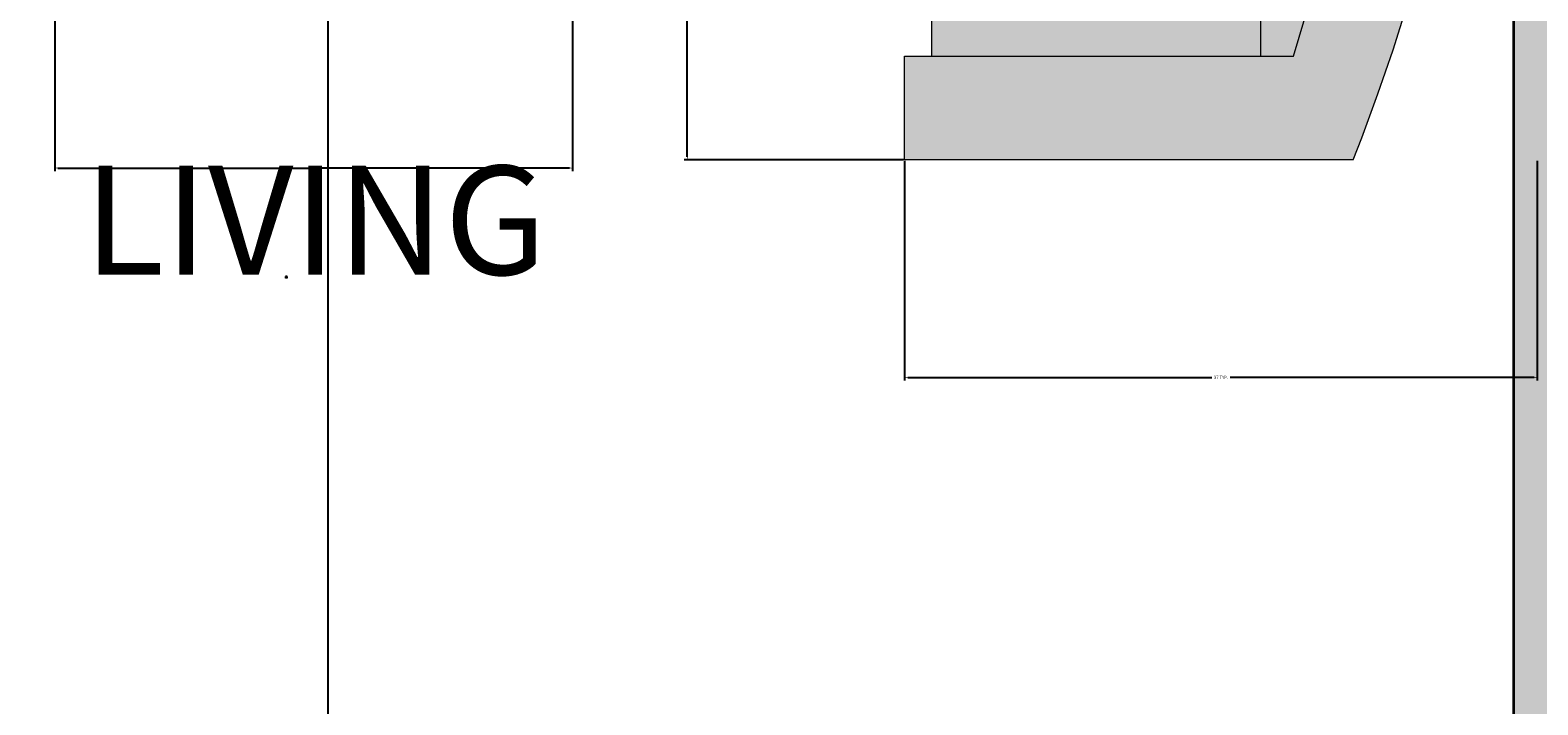
# Model space of a CAD drawing. Units: inches. Extents: x 2549 to 3108, y 1683 to 2362.
# Tile 23 of 30: x 2949 to 3036, y 1979 to 2018. Entities that reach past the tile are written whole.
import ezdxf

# ---------------------------------------------------------------- set-up
doc = ezdxf.new("R2010")
doc.units = ezdxf.units.IN
for name, color, linetype, lineweight in [('A-ANNO-DIMS', 2, 'Continuous', 18), ('A-AREA-IDEN', 7, 'Continuous', 18), ('A-FURN', 8, 'Continuous', 18), ('A-FURN-PATT', 9, 'Continuous', 13), ('A-WALL', 7, 'Continuous', 35), ('A-WALL-PATT', 89, 'Continuous', 13)]:
    doc.layers.add(name, color=color, linetype=linetype, lineweight=lineweight)
doc.layers.add('C-PKNG-VEHI-PATT', color=251, linetype='Continuous', lineweight=13, true_color=0x636466)
doc.layers.add('C-PVMT-PATT', color=9, linetype='Continuous', lineweight=13, true_color=0xc7c8ca)
doc.styles.get("Standard").update_dxf_attribs({"font": 'arial.ttf'})
doc.dimstyles.get("Standard").update_dxf_attribs({"dimtxt": 0.18, "dimasz": 0.18, "dimexe": 0.18, "dimexo": 0.0625, "dimgap": 0.09, "dimtad": 0, "dimtih": 1, "dimtoh": 1, "dimdec": 4, "dimzin": 0, "dimdsep": 46, "dimtxsty": 'Standard', "dimcen": 0.09, "dimadec": 0, "dimazin": 0, "dimtfac": 1, "dimtdec": 4, "dimtofl": 0, "dimtmove": 0, "dimatfit": 3, "dimfxl": 1, "dimtolj": 1, "dimtzin": 0, "dimarcsym": 0})

# ---------------------------------------------------------------- blocks, each defined once
blk = doc.blocks.new('Sofa - Roundback 7 ft.')
for p, q in [((-12.00002, -32.4421), (-12.00003, -6.5971)), ((11.99997, -32.4421), (11.99998, -6.5971)), ((-36.000027, -34), (-36.000027, -11.4696)), ((35.99998, -34), (35.99998, -11.4696)), ((-35.999844, -13.3819), (35.9998, -13.3819)), ((-36.000027, -32.4421), (35.99998, -32.4421))]:
    blk.add_line(p, q)
for points in [[(-36.000027, -34), (-42.000027, -34), (-42.000027, -8)], [(41.99998, -8), (41.99998, -34), (35.99998, -34)]]:
    blk.add_lwpolyline(points)
for centre, radius, start, end in [((0, -114.25), 114.25, 68.43141, 111.5686), ((-0.00001, -127.1968), 121.1968, 72.72033, 107.2797)]:
    blk.add_arc(centre, radius, start, end)
blk = doc.blocks.new('*D16')
at = {"layer": 'A-ANNO-DIMS', "color": 0, "lineweight": -2, "transparency": 16777216}
for p, q in [((2999.284, 2094.091), (2986.567, 2094.091)), ((2986.747, 2093.911), (2986.747, 2052.274)), ((2986.747, 2010.271), (2986.747, 2051.907)), ((2999.284, 2010.091), (2986.567, 2010.091))]:
    blk.add_line(p, q, dxfattribs=at)
at = {"layer": 'A-ANNO-DIMS', "color": 0, "transparency": 16777216}
for points in [[(2986.717, 2093.911), (2986.777, 2093.911), (2986.747, 2094.091)], [(2986.717, 2010.271), (2986.777, 2010.271), (2986.747, 2010.091)]]:
    blk.add_solid(points, dxfattribs=at)
at = {"layer": 'Defpoints', "color": 0, "transparency": 16777216}
for p in [(2999.347, 2094.091), (2986.747, 2010.091), (2999.347, 2010.091)]:
    blk.add_point(p, dxfattribs=at)
at = {"layer": 'A-ANNO-DIMS', "color": 0, "transparency": 16777216, "insert": (2986.747, 2052.091), "char_height": 0.18, "attachment_point": 5}
blk.add_mtext('\\A1;SOFA 84 TYP.', dxfattribs=at)
blk = doc.blocks.new('*D17')
at = {"layer": 'A-ANNO-DIMS', "color": 0, "lineweight": -2, "transparency": 16777216}
for p, q in [((2999.347, 2010.028), (2999.347, 1997.311)), ((3036.014, 2010.028), (3036.014, 1997.311)), ((2999.527, 1997.491), (3017.152, 1997.491)), ((3035.834, 1997.491), (3018.208, 1997.491))]:
    blk.add_line(p, q, dxfattribs=at)
at = {"layer": 'A-ANNO-DIMS', "color": 0, "transparency": 16777216}
for points in [[(2999.527, 1997.521), (2999.527, 1997.461), (2999.347, 1997.491)], [(3035.834, 1997.521), (3035.834, 1997.461), (3036.014, 1997.491)]]:
    blk.add_solid(points, dxfattribs=at)
at = {"layer": 'Defpoints', "color": 0, "transparency": 16777216}
for p in [(2999.347, 2010.091), (3036.014, 2010.091), (3036.014, 1997.491)]:
    blk.add_point(p, dxfattribs=at)
at = {"layer": 'A-ANNO-DIMS', "color": 0, "transparency": 16777216, "insert": (3017.68, 1997.491), "char_height": 0.18, "attachment_point": 5}
blk.add_mtext('\\A1;37 TYP.', dxfattribs=at)
blk = doc.blocks.new('*D23')
at = {"layer": 'A-ANNO-DIMS', "color": 0, "lineweight": -2, "transparency": 16777216}
for p, q in [((2950.093, 2018.552), (2950.093, 2009.435)), ((2980.093, 2018.552), (2980.093, 2009.435)), ((2950.273, 2009.615), (2964.875, 2009.615)), ((2979.913, 2009.615), (2965.312, 2009.615))]:
    blk.add_line(p, q, dxfattribs=at)
at = {"layer": 'A-ANNO-DIMS', "color": 0, "transparency": 16777216}
for points in [[(2950.273, 2009.645), (2950.273, 2009.585), (2950.093, 2009.615)], [(2979.913, 2009.645), (2979.913, 2009.585), (2980.093, 2009.615)]]:
    blk.add_solid(points, dxfattribs=at)
at = {"layer": 'Defpoints', "color": 0, "transparency": 16777216}
for p in [(2950.093, 2018.615), (2980.093, 2018.615), (2980.093, 2009.615)]:
    blk.add_point(p, dxfattribs=at)
at = {"layer": 'A-ANNO-DIMS', "color": 0, "transparency": 16777216, "insert": (2965.093, 2009.615), "char_height": 0.18, "attachment_point": 5}
blk.add_mtext('\\A1;30', dxfattribs=at)
blk = doc.blocks.new('*D46')
at = {"layer": 'A-ANNO-DIMS', "color": 0, "lineweight": -2, "transparency": 16777216}
for p, q in [((2812.643, 2140.461), (2812.643, 1683.444)), ((3034.643, 2134.461), (3034.643, 1683.444)), ((2812.823, 1683.624), (2923.353, 1683.624)), ((3034.463, 1683.624), (2923.932, 1683.624))]:
    blk.add_line(p, q, dxfattribs=at)
at = {"layer": 'A-ANNO-DIMS', "color": 0, "transparency": 16777216}
for points in [[(2812.823, 1683.654), (2812.823, 1683.594), (2812.643, 1683.624)], [(3034.463, 1683.654), (3034.463, 1683.594), (3034.643, 1683.624)]]:
    blk.add_solid(points, dxfattribs=at)
at = {"layer": 'Defpoints', "color": 0, "transparency": 16777216}
for p in [(2812.643, 2140.524), (3034.643, 2134.524), (3034.643, 1683.624)]:
    blk.add_point(p, dxfattribs=at)
at = {"layer": 'A-ANNO-DIMS', "color": 0, "transparency": 16777216, "insert": (2923.643, 1683.624), "char_height": 0.18, "attachment_point": 5}
blk.add_mtext('\\A1;222', dxfattribs=at)
blk = doc.blocks.new('*D57')
at = {"layer": 'A-ANNO-DIMS', "color": 0, "lineweight": -2, "transparency": 16777216}
for p, q in [((2965.935, 1936.586), (2965.935, 2362.323)), ((2966.115, 2362.143), (2999.912, 2362.143)), ((3034.463, 2362.143), (3000.666, 2362.143)), ((3034.643, 1936.586), (3034.643, 2362.323))]:
    blk.add_line(p, q, dxfattribs=at)
at = {"layer": 'A-ANNO-DIMS', "color": 0, "transparency": 16777216}
for points in [[(2966.115, 2362.173), (2966.115, 2362.113), (2965.935, 2362.143)], [(3034.463, 2362.173), (3034.463, 2362.113), (3034.643, 2362.143)]]:
    blk.add_solid(points, dxfattribs=at)
at = {"layer": 'Defpoints', "color": 0, "transparency": 16777216}
for p in [(3034.643, 2362.143), (2965.935, 1936.524), (3034.643, 1936.524)]:
    blk.add_point(p, dxfattribs=at)
at = {"layer": 'A-ANNO-DIMS', "color": 0, "transparency": 16777216, "insert": (3000.289, 2362.143), "char_height": 0.18, "attachment_point": 5}
blk.add_mtext('\\A1;68.71', dxfattribs=at)
blk = doc.blocks.new('*D63')
at = {"layer": 'A-ANNO-DIMS', "color": 0, "lineweight": -2, "transparency": 16777216}
for p, q in [((2963.328, 2197.213), (2963.508, 2197.213)), ((2963.508, 2197.213), (2963.508, 2124.675)), ((2963.419, 2003.299), (2963.599, 2003.299)), ((2963.509, 2003.209), (2963.509, 2003.389))]:
    blk.add_line(p, q, dxfattribs=at)
at = {"layer": 'A-ANNO-DIMS', "color": 0, "transparency": 16777216}
blk.add_solid([(2963.538, 2124.675), (2963.478, 2124.675), (2963.508, 2124.495)], dxfattribs=at)
at = {"layer": 'Defpoints', "color": 0, "transparency": 16777216}
for p in [(2963.508, 2124.495), (2963.509, 2003.299)]:
    blk.add_point(p, dxfattribs=at)
at = {"layer": 'A-ANNO-DIMS', "color": 0, "transparency": 16777216, "insert": (2962.654, 2197.213), "char_height": 0.18, "attachment_point": 5}
blk.add_mtext('\\A1;2X R121.2', dxfattribs=at)

msp = doc.modelspace()

# ---------------------------------------------------------------- hatches: boundary and pattern name
at = {"layer": 'A-FURN-PATT', "transparency": 33554567}
h = msp.add_hatch(color=256, dxfattribs=at)
h.dxf.hatch_style = 1
h.paths.add_polyline_path([(2708.7147, 2271.6737), (2675.2813, 2271.6737), (2675.2813, 2262.0404), (2708.7147, 2262.0404)])
h.paths.add_polyline_path([(2980.8246, 2271.6737), (2947.3913, 2271.6737), (2947.3913, 2262.0404), (2980.8246, 2262.0404)])
h.paths.add_polyline_path([(2748.8496, 2101.6383), (2798.148, 2101.6383), (2798.148, 2111.4248), (2748.8496, 2111.4248)], flags=9)
h.paths.add_polyline_path([(2685.2081, 2101.489), (2719.3253, 2101.489), (2719.3253, 2111.2819), (2685.2081, 2111.2819)], flags=9)
h.paths.add_polyline_path([(2814.6852, 1907.1328), (2847.8384, 1907.1328), (2847.8384, 1916.9258), (2814.6852, 1916.9258)], flags=9)
h.paths.add_polyline_path([(2814.3906, 1835.5864), (2848.0172, 1835.5864), (2848.0172, 1845.3794), (2814.3906, 1845.3794)], flags=9)
h.paths.add_polyline_path([(2800.5245, 1759.1674), (2853.7435, 1759.1674), (2853.7435, 1768.954), (2800.5245, 1768.954)], flags=9)
h.paths.add_polyline_path([(2972.4611, 1807.3305), (3015.3943, 1807.3305), (3015.3943, 1817.117), (2972.4611, 1817.117)], flags=9)
h.paths.add_polyline_path([(2902.3327, 1888.6731), (2937.9131, 1888.6731), (2937.9131, 1898.4661), (2902.3327, 1898.4661)], flags=9)
h.paths.add_polyline_path([(2712.1779, 1878.9039), (2754.1257, 1878.9039), (2754.1257, 1888.6904), (2712.1779, 1888.6904)], flags=9)
h.paths.add_polyline_path([(2614.0056, 2012.812), (2650.0251, 2012.812), (2650.0251, 2022.4371), (2614.0056, 2022.4371)], flags=9)
h.paths.add_polyline_path([(2713.3129, 2003.1645), (2747.4237, 2003.1645), (2747.4237, 2012.951), (2713.3129, 2012.951)], flags=9)
h.paths.add_polyline_path([(2950.1379, 2001.6934), (2982.2992, 2001.6934), (2982.2992, 2011.48), (2950.1379, 2011.48)], flags=9)
h.paths.add_polyline_path([(2940.864, 2238.5537), (2997.5066, 2238.5537), (2997.5066, 2248.3466), (2940.864, 2248.3466)], flags=9)
h.paths.add_polyline_path([(2821.5457, 2202.8348), (2855.663, 2202.8348), (2855.663, 2212.6278), (2821.5457, 2212.6278)], flags=9)
h.paths.add_polyline_path([(2661.8026, 2238.6249), (2718.4451, 2238.6249), (2718.4451, 2248.4179), (2661.8026, 2248.4179)], flags=9)
h = msp.add_hatch(color=256, dxfattribs=at)
h.dxf.hatch_style = 1
h.paths.add_polyline_path([(2906.5064, 1905.2148), (2905.2584, 1904.3827), (2907.0611, 1900.7772), (2908.3092, 1901.6092)])
h.paths.add_polyline_path([(2936.522, 1914.8044), (2935.2739, 1915.6364), (2932.6391, 1912.5856), (2933.8871, 1911.7535)])
h.paths.add_polyline_path([(2950.2508, 1905.6518), (2949.0027, 1906.4839), (2947.1999, 1902.8783), (2948.448, 1902.0463)])
h.paths.add_polyline_path([(2958.5713, 1918.1326), (2956.9072, 1919.242), (2952.4696, 1908.98, 1.3874274), (2954.9657, 1907.3159)])
h.paths.add_polyline_path([(2945.2585, 1927.0078), (2943.5944, 1928.1172), (2934.9965, 1920.6287, 1.3874274), (2937.4927, 1918.9646)])
h.paths.add_polyline_path([(2748.8496, 2101.6383), (2798.148, 2101.6383), (2798.148, 2111.4248), (2748.8496, 2111.4248)], flags=9)
h.paths.add_polyline_path([(2685.2081, 2101.489), (2719.3253, 2101.489), (2719.3253, 2111.2819), (2685.2081, 2111.2819)], flags=9)
h.paths.add_polyline_path([(2814.6852, 1907.1328), (2847.8384, 1907.1328), (2847.8384, 1916.9258), (2814.6852, 1916.9258)], flags=9)
h.paths.add_polyline_path([(2814.3906, 1835.5864), (2848.0172, 1835.5864), (2848.0172, 1845.3794), (2814.3906, 1845.3794)], flags=9)
h.paths.add_polyline_path([(2800.5245, 1759.1674), (2853.7435, 1759.1674), (2853.7435, 1768.954), (2800.5245, 1768.954)], flags=9)
h.paths.add_polyline_path([(2972.4611, 1807.3305), (3015.3943, 1807.3305), (3015.3943, 1817.117), (2972.4611, 1817.117)], flags=9)
h.paths.add_polyline_path([(2902.3327, 1888.6731), (2937.9131, 1888.6731), (2937.9131, 1898.4661), (2902.3327, 1898.4661)], flags=9)
h.paths.add_polyline_path([(2712.1779, 1878.9039), (2754.1257, 1878.9039), (2754.1257, 1888.6904), (2712.1779, 1888.6904)], flags=9)
h.paths.add_polyline_path([(2614.0056, 2012.812), (2650.0251, 2012.812), (2650.0251, 2022.4371), (2614.0056, 2022.4371)], flags=9)
h.paths.add_polyline_path([(2713.3129, 2003.1645), (2747.4237, 2003.1645), (2747.4237, 2012.951), (2713.3129, 2012.951)], flags=9)
h.paths.add_polyline_path([(2950.1379, 2001.6934), (2982.2992, 2001.6934), (2982.2992, 2011.48), (2950.1379, 2011.48)], flags=9)
h.paths.add_polyline_path([(2940.864, 2238.5537), (2997.5066, 2238.5537), (2997.5066, 2248.3466), (2940.864, 2248.3466)], flags=9)
h.paths.add_polyline_path([(2821.5457, 2202.8348), (2855.663, 2202.8348), (2855.663, 2212.6278), (2821.5457, 2212.6278)], flags=9)
h.paths.add_polyline_path([(2661.8026, 2238.6249), (2718.4451, 2238.6249), (2718.4451, 2248.4179), (2661.8026, 2248.4179)], flags=9)
at = {"layer": 'A-FURN-PATT', "transparency": 33554684}
h = msp.add_hatch(color=256, dxfattribs=at)
h.dxf.hatch_style = 1
h.paths.add_polyline_path([(2927.5085, 2119.0252, -0.1519478), (2999.5085, 2119.0252), (2999.5085, 2096.4953), (3005.5085, 2096.4953), (3005.5085, 2122.4953, 0.1904762), (2921.5085, 2122.4953), (2921.5085, 2096.4953), (2927.5085, 2096.4953)])
h.paths.add_polyline_path([(2951.5085, 2117.1134), (2927.5085, 2117.1134), (2927.5085, 2098.0532), (2951.5085, 2098.0532)], flags=17)
h.paths.add_polyline_path([(2975.5085, 2117.1134), (2951.5085, 2117.1134), (2951.5085, 2098.0532), (2975.5085, 2098.0532)], flags=17)
h.paths.add_polyline_path([(2975.5085, 2123.8998, 0.0496282), (2951.5085, 2123.8998), (2951.5085, 2117.1134), (2975.5085, 2117.1134)], flags=17)
h.paths.add_polyline_path([(2951.5085, 2123.8998, 0.0506466), (2927.5085, 2119.0252), (2927.5085, 2117.1134), (2951.5085, 2117.1134)], flags=17)
h.paths.add_polyline_path([(2975.5085, 2123.8998), (2975.5085, 2117.1134), (2999.5085, 2117.1134), (2999.5085, 2119.0252, 0.0506467)], flags=17)
h.paths.add_polyline_path([(2999.5085, 2117.1134), (2975.5085, 2117.1134), (2975.5085, 2098.0532), (2999.5085, 2098.0532)], flags=17)
h.paths.add_polyline_path([(3019.9651, 2088.0905), (3000.9049, 2088.0905), (3000.9049, 2064.0905), (3019.9651, 2064.0905)], flags=17)
h.paths.add_polyline_path([(3025.347, 2094.0905), (2999.347, 2094.0905), (2999.347, 2088.0905), (3021.8769, 2088.0905, -0.1519478), (3021.8769, 2016.0905), (2999.347, 2016.0905), (2999.347, 2010.0905), (3025.347, 2010.0905, 0.1904762)])
h.paths.add_polyline_path([(3021.8769, 2088.0905), (3019.9651, 2088.0905), (3019.9651, 2064.0905), (3026.7514, 2064.0905, 0.0506466)], flags=17)
h.paths.add_polyline_path([(3026.7514, 2064.0905), (3019.9651, 2064.0905), (3019.9651, 2040.0905), (3026.7514, 2040.0905, 0.0496282)], flags=17)
h.paths.add_polyline_path([(3019.9651, 2064.0905), (3000.9049, 2064.0905), (3000.9049, 2040.0905), (3019.9651, 2040.0905)], flags=17)
h.paths.add_polyline_path([(3019.9651, 2040.0905), (3000.9049, 2040.0905), (3000.9049, 2016.0905), (3019.9651, 2016.0905)], flags=17)
h.paths.add_polyline_path([(3026.7514, 2040.0905), (3019.9651, 2040.0905), (3019.9651, 2016.0905), (3021.8769, 2016.0905, 0.0506467)], flags=17)
at = {"layer": 'A-WALL-PATT'}
h = msp.add_hatch(color=256, dxfattribs=at)
h.dxf.hatch_style = 1
h.paths.add_polyline_path([(2638.6427, 2272.5237), (3034.6427, 2272.5237), (3034.6427, 1936.5237), (3043.6427, 1936.5237), (3043.6427, 2281.5237), (2629.6427, 2281.5237), (2629.6427, 2074.5237), (2812.6427, 2074.5237), (2812.6427, 2140.5237), (2785.7177, 2140.5237), (2785.7177, 2134.5237), (2806.6427, 2134.5237), (2806.6427, 2080.5237), (2638.6427, 2080.5237)])
h.paths.add_polyline_path([(2638.6427, 1972.5237), (2662.6427, 1972.5237), (2662.6427, 2041.0557), (2653.6427, 2041.0557), (2653.6427, 1978.5237), (2629.6427, 1978.5237), (2629.6427, 1795.5237), (2662.6427, 1795.5237), (2881.6427, 1795.5237), (2881.6427, 1936.5237), (2965.9351, 1936.5237), (2965.9351, 1974.5439), (2959.9351, 1974.5439), (2959.9351, 1945.5237), (2881.6427, 1945.5237), (2872.6427, 1945.5237), (2872.6427, 1804.5237), (2662.6427, 1804.5237), (2638.6427, 1804.5237)])
at = {"layer": 'C-PKNG-VEHI-PATT'}
h = msp.add_hatch(color=256, dxfattribs=at)
h.dxf.hatch_style = 1
edge = h.paths.add_edge_path()
edge.add_ellipse((2935.7258, 1791.964), major_axis=(-50.66, 0), ratio=0.8423039, start_angle=248.165046, end_angle=265.722579)
edge.add_line((2938.911, 1834.5507), (2925.8653, 1834.5507))
edge.add_ellipse((2929.0505, 1791.964), major_axis=(50.66, 0), ratio=0.8423039, start_angle=94.277421, end_angle=111.834954)
edge.add_line((2912.8508, 1832.3947), (2914.2044, 1822.2495))
edge.add_ellipse((2930.6538, 1783.1023), major_axis=(-49.3014, 0), ratio=0.8423039, start_angle=-85.12993, end_angle=-67.208085, ccw=False)
edge.add_line((2927.1247, 1824.5225), (2937.6516, 1824.5225))
edge.add_ellipse((2934.1225, 1783.1023), major_axis=(49.3014, 0), ratio=0.8423039, start_angle=67.208085, end_angle=85.12993, ccw=False)
edge.add_line((2950.5719, 1822.2495), (2951.9255, 1832.3947))
edge = h.paths.add_edge_path()
edge.add_ellipse((2903.4793, 1857.3351), major_axis=(-34.7979, 0), ratio=0.8423039, start_angle=180, end_angle=209.43857)
edge.add_ellipse((2961.297, 1857.3351), major_axis=(34.7979, 0), ratio=0.8423039, start_angle=150.56143, end_angle=180)
edge.add_line((2926.4991, 1857.3351), (2926.4991, 1843.7609))
edge.add_ellipse((2924.1251, 1844.3143), major_axis=(-0.2209, 3.9278), ratio=0.6038336, start_angle=89.002014, end_angle=253.657408, ccw=False)
edge.add_line((2921.7512, 1844.2222), (2921.7512, 1853.3975))
edge.add_line((2921.7512, 1853.3975), (2925.269, 1855.8484))
edge.add_ellipse((2925.4782, 1855.4931), major_axis=(0.4584, 0), ratio=0.8423039, start_angle=90, end_angle=134.480211, ccw=False)
edge.add_line((2925.4782, 1855.8792), (2926.4991, 1855.8792))
edge.add_line((2926.4991, 1855.8792), (2926.4991, 1857.3351))
edge.add_ellipse((2961.297, 1857.3351), major_axis=(34.7979, 0), ratio=0.8423039, start_angle=150.56143, end_angle=180, ccw=False)
edge.add_line((2932.3882, 1873.6501), (2932.3882, 1875.7801))
edge.add_ellipse((2932.3882, 1875.3939), major_axis=(0.4584, 0), ratio=0.8423039, start_angle=90, end_angle=127.93313)
edge.add_line((2932.1366, 1875.7167), (2928.5915, 1873.7564))
edge.add_ellipse((2899.9271, 2002.4692), major_axis=(155.4756, 0), ratio=0.84230387, start_angle=-80.743434, end_angle=-77.445067, ccw=False)
edge.add_ellipse((2949.4402, 1715.2151), major_axis=(-189.1422, 0), ratio=0.84230387, start_angle=-79.790461, end_angle=-77.555373)
edge.add_ellipse((3300.3614, 1852.5642), major_axis=(-386.1662, 0), ratio=0.84230387, start_angle=-2.863715, end_angle=2.198541)
edge.add_ellipse((2929.0505, 1792.5159), major_axis=(-55.6192, 0), ratio=0.8423039, start_angle=-85.917589, end_angle=-72.280047, ccw=False)
edge.add_line((2925.7129, 1839.2798), (2939.0634, 1839.2798))
edge.add_ellipse((2935.7258, 1792.5159), major_axis=(55.6192, 0), ratio=0.8423039, start_angle=72.280047, end_angle=85.917589, ccw=False)
edge.add_ellipse((2564.4149, 1852.5642), major_axis=(-386.1662, 0), ratio=0.84230387, start_angle=177.801459, end_angle=182.863715)
edge.add_ellipse((2915.3361, 1715.2151), major_axis=(189.1422, 0), ratio=0.84230387, start_angle=77.555373, end_angle=79.790461)
edge.add_ellipse((2964.8492, 2002.4692), major_axis=(-155.4756, 0), ratio=0.84230387, start_angle=77.445067, end_angle=80.743434, ccw=False)
edge.add_line((2936.1848, 1873.7564), (2932.6397, 1875.7167))
edge.add_ellipse((2932.3882, 1875.3939), major_axis=(0.4584, 0), ratio=0.8423039, start_angle=52.06687, end_angle=90)
edge.add_line((2932.3882, 1875.7801), (2932.3882, 1873.6501))
edge.add_ellipse((2903.4793, 1857.3351), major_axis=(-34.7979, 0), ratio=0.8423039, start_angle=180, end_angle=209.43857, ccw=False)
edge.add_line((2938.2772, 1857.3351), (2938.2772, 1855.8792))
edge.add_line((2938.2772, 1855.8792), (2939.4059, 1855.8792))
edge.add_ellipse((2939.2981, 1855.4931), major_axis=(-0.4584, 0), ratio=0.8423039, start_angle=225.519789, end_angle=270, ccw=False)
edge.add_line((2939.5903, 1855.7906), (2943.0251, 1853.3975))
edge.add_line((2943.0251, 1853.3975), (2943.0251, 1844.2222))
edge.add_ellipse((2940.6512, 1844.3143), major_axis=(0.2209, 3.9278), ratio=0.6038336, start_angle=106.342592, end_angle=270.997986, ccw=False)
edge.add_line((2938.2772, 1843.7609), (2938.2772, 1857.3351))
edge = h.paths.add_edge_path()
edge.add_ellipse((2932.3882, 1865.1973), major_axis=(91.081, 0), ratio=0.8423039, start_angle=256.401865, end_angle=283.598135, ccw=False)
edge.add_line((2914.2044, 1790.0239), (2914.2044, 1778.3622))
edge.add_ellipse((2932.3882, 1853.5356), major_axis=(91.081, 0), ratio=0.8423039, start_angle=256.401865, end_angle=283.598135)
edge.add_line((2950.5719, 1778.3622), (2950.5719, 1790.0239))
edge = h.paths.add_edge_path()
edge.add_ellipse((2948.7383, 1772.3145), major_axis=(1.8336, 0), ratio=0.8423039, start_angle=0, end_angle=90)
edge.add_line((2948.7383, 1773.859), (2916.038, 1773.859))
edge.add_ellipse((2916.038, 1772.3145), major_axis=(1.8336, 0), ratio=0.8423039, start_angle=90, end_angle=180)
edge.add_line((2914.2044, 1772.3145), (2914.2044, 1760.2558))
edge.add_line((2914.2044, 1760.2558), (2950.5719, 1760.2558))
edge.add_line((2950.5719, 1760.2558), (2950.5719, 1772.3145))
h.paths.add_polyline_path([(2748.8496, 2101.6383), (2798.148, 2101.6383), (2798.148, 2111.4248), (2748.8496, 2111.4248)], flags=9)
h.paths.add_polyline_path([(2685.2081, 2101.489), (2719.3253, 2101.489), (2719.3253, 2111.2819), (2685.2081, 2111.2819)], flags=9)
h.paths.add_polyline_path([(2814.6852, 1907.1328), (2847.8384, 1907.1328), (2847.8384, 1916.9258), (2814.6852, 1916.9258)], flags=9)
h.paths.add_polyline_path([(2814.3906, 1835.5864), (2848.0172, 1835.5864), (2848.0172, 1845.3794), (2814.3906, 1845.3794)], flags=9)
h.paths.add_polyline_path([(2800.5245, 1759.1674), (2853.7435, 1759.1674), (2853.7435, 1768.954), (2800.5245, 1768.954)], flags=9)
h.paths.add_polyline_path([(2972.4611, 1807.3305), (3015.3943, 1807.3305), (3015.3943, 1817.117), (2972.4611, 1817.117)], flags=9)
h.paths.add_polyline_path([(2902.3327, 1888.6731), (2937.9131, 1888.6731), (2937.9131, 1898.4661), (2902.3327, 1898.4661)], flags=9)
h.paths.add_polyline_path([(2712.1779, 1878.9039), (2754.1257, 1878.9039), (2754.1257, 1888.6904), (2712.1779, 1888.6904)], flags=9)
h.paths.add_polyline_path([(2614.0056, 2012.812), (2650.0251, 2012.812), (2650.0251, 2022.4371), (2614.0056, 2022.4371)], flags=9)
h.paths.add_polyline_path([(2713.3129, 2003.1645), (2747.4237, 2003.1645), (2747.4237, 2012.951), (2713.3129, 2012.951)], flags=9)
h.paths.add_polyline_path([(2950.1379, 2001.6934), (2982.2992, 2001.6934), (2982.2992, 2011.48), (2950.1379, 2011.48)], flags=9)
h.paths.add_polyline_path([(2940.864, 2238.5537), (2997.5066, 2238.5537), (2997.5066, 2248.3466), (2940.864, 2248.3466)], flags=9)
h.paths.add_polyline_path([(2821.5457, 2202.8348), (2855.663, 2202.8348), (2855.663, 2212.6278), (2821.5457, 2212.6278)], flags=9)
h.paths.add_polyline_path([(2661.8026, 2238.6249), (2718.4451, 2238.6249), (2718.4451, 2248.4179), (2661.8026, 2248.4179)], flags=9)
at = {"layer": 'C-PVMT-PATT'}
h = msp.add_hatch(color=256, dxfattribs=at)
h.dxf.hatch_style = 1
h.paths.add_polyline_path([(3067.6427, 2305.5237), (2605.6427, 2305.5237), (2605.6427, 2074.5237), (2629.6427, 2074.5237), (2629.6427, 2281.5237), (3043.6427, 2281.5237), (3043.6427, 1885.5237), (3043.6427, 1872.8745), (3031.1672, 1872.8745), (3031.1672, 1862.5731), (2995.8054, 1862.5731), (2995.8054, 1872.8745), (2983.1752, 1872.8745), (2983.1752, 1885.5237), (2881.6427, 1885.5237), (2881.6427, 1795.5237), (2751.0977, 1795.5237), (2751.0977, 1761.5237), (2786.1577, 1761.5237), (2786.1577, 1723.5237), (2881.84, 1723.5237), (2881.84, 1714.5237), (3067.6427, 1714.5237), (3067.6427, 1723.5237)])
edge = h.paths.add_edge_path(flags=16)
edge.add_ellipse((2949.4402, 1710.9683), major_axis=(-194.1014, 0), ratio=0.84230387, start_angle=-77.874034, end_angle=-76.219471, ccw=False)
edge.add_ellipse((2949.4402, 1715.2151), major_axis=(-189.1422, 0), ratio=0.84230387, start_angle=-79.790461, end_angle=-77.555373, ccw=False)
edge.add_ellipse((2899.9271, 2002.4692), major_axis=(155.4756, 0), ratio=0.84230387, start_angle=-80.743434, end_angle=-77.445067)
edge.add_line((2928.5915, 1873.7564), (2932.3882, 1875.8558))
edge.add_line((2932.3882, 1875.8558), (2936.1848, 1873.7564))
edge.add_ellipse((2964.8492, 2002.4692), major_axis=(-155.4756, 0), ratio=0.84230387, start_angle=77.445067, end_angle=80.743434)
edge.add_ellipse((2915.3361, 1715.2151), major_axis=(189.1422, 0), ratio=0.84230387, start_angle=77.555373, end_angle=79.790461, ccw=False)
edge.add_ellipse((2915.3361, 1710.9683), major_axis=(-194.1014, 0), ratio=0.84230387, start_angle=256.219471, end_angle=257.874034, ccw=False)
edge.add_ellipse((2628.2871, 1850.2612), major_axis=(-327.2532, 0), ratio=0.84230387, start_angle=182.17995, end_angle=183.650428, ccw=False)
edge.add_ellipse((2955.5637, 1861.9334), major_axis=(-0.9168, 0), ratio=0.8423039, start_angle=180, end_angle=270, ccw=False)
edge.add_line((2956.4805, 1862.3857), (2956.4805, 1846.4866))
edge.add_ellipse((2955.5637, 1846.939), major_axis=(-0.9168, 0), ratio=0.8423039, start_angle=90, end_angle=180, ccw=False)
edge.add_ellipse((-3607.0606, 1835.832), major_axis=(-6562.6242, 0), ratio=0.84230387, start_angle=179.61613322, end_angle=180.09022909, ccw=False)
edge.add_ellipse((2955.5637, 1791.0926), major_axis=(0.9168, 0), ratio=0.8423039, start_angle=0, end_angle=90, ccw=False)
edge.add_line((2956.4805, 1791.545), (2956.4805, 1775.6459))
edge.add_ellipse((2955.5637, 1776.0982), major_axis=(0.9168, 0), ratio=0.8423039, start_angle=270, end_angle=360, ccw=False)
edge.add_ellipse((-3607.0606, 1835.832), major_axis=(-6562.6242, 0), ratio=0.84230387, start_angle=179.3813568, end_angle=179.47172853, ccw=False)
edge.add_ellipse((2954.5907, 1763.8768), major_axis=(-1.3752, 0), ratio=0.8423039, start_angle=179.371763, end_angle=248.464757, ccw=False)
edge.add_ellipse((-3607.519, 1835.832), major_axis=(-6564.0409, 0), ratio=0.842303863, start_angle=179.35344594, end_angle=179.37176282, ccw=False)
edge.add_ellipse((2952.6829, 1761.8002), major_axis=(3.2503, 0), ratio=0.8423039, start_angle=-90, end_angle=-0.646554, ccw=False)
edge.add_line((2952.6829, 1759.0625), (2912.0934, 1759.0625))
edge.add_ellipse((2912.0934, 1761.8002), major_axis=(3.2503, 0), ratio=0.8423039, start_angle=180.646554, end_angle=270, ccw=False)
edge.add_ellipse((9472.2953, 1835.832), major_axis=(-6564.0409, 0), ratio=0.842303871, start_angle=0.62823722, end_angle=0.6465541, ccw=False)
edge.add_ellipse((2910.1856, 1763.8768), major_axis=(1.3752, 0), ratio=0.8423039, start_angle=111.535244, end_angle=180.628237, ccw=False)
edge.add_ellipse((9471.8369, 1835.832), major_axis=(-6562.6242, 0), ratio=0.84230387, start_angle=0.52827147, end_angle=0.6465541, ccw=False)
edge.add_ellipse((2909.2126, 1776.0982), major_axis=(-0.9168, 0), ratio=0.8423039, start_angle=0, end_angle=90, ccw=False)
edge.add_line((2908.2958, 1775.6459), (2908.2958, 1791.545))
edge.add_ellipse((2909.2126, 1791.0926), major_axis=(-0.9168, 0), ratio=0.8423039, start_angle=-90, end_angle=0, ccw=False)
edge.add_ellipse((9471.8369, 1835.832), major_axis=(-6562.6242, 0), ratio=0.84230387, start_angle=-0.09022909, end_angle=0.38386678, ccw=False)
edge.add_ellipse((2909.2126, 1846.939), major_axis=(-0.9168, 0), ratio=0.8423039, start_angle=0, end_angle=90, ccw=False)
edge.add_line((2908.2958, 1846.4866), (2908.2958, 1862.3857))
edge.add_ellipse((2909.2126, 1861.9334), major_axis=(0.9168, 0), ratio=0.8423039, start_angle=90, end_angle=180, ccw=False)
edge.add_ellipse((3236.4892, 1850.2612), major_axis=(327.2532, 0), ratio=0.84230387, start_angle=176.349572, end_angle=177.82005, ccw=False)
edge = h.paths.add_edge_path(flags=0)
edge.add_ellipse((2903.4793, 1857.3351), major_axis=(-34.7979, 0), ratio=0.8423039, start_angle=180, end_angle=209.43857, ccw=False)
edge.add_line((2938.2772, 1857.3351), (2938.2772, 1855.8792))
edge.add_line((2938.2772, 1855.8792), (2939.4631, 1855.8792))
edge.add_line((2939.4631, 1855.8792), (2943.0251, 1853.3975))
edge.add_line((2943.0251, 1853.3975), (2943.0251, 1844.2222))
edge.add_ellipse((2940.6512, 1844.3143), major_axis=(0.2209, 3.9278), ratio=0.6038336, start_angle=106.342592, end_angle=270.997986, ccw=False)
edge.add_line((2938.2772, 1843.7609), (2938.2772, 1857.3351))
edge.add_ellipse((2903.4793, 1857.3351), major_axis=(-34.7979, 0), ratio=0.8423039, start_angle=180, end_angle=209.43857)
edge.add_ellipse((2961.297, 1857.3351), major_axis=(34.7979, 0), ratio=0.8423039, start_angle=150.56143, end_angle=180)
edge.add_line((2926.4991, 1857.3351), (2926.4991, 1843.7609))
edge.add_ellipse((2924.1251, 1844.3143), major_axis=(-0.2209, 3.9278), ratio=0.6038336, start_angle=89.002014, end_angle=253.657408, ccw=False)
edge.add_line((2921.7512, 1844.2222), (2921.7512, 1853.3975))
edge.add_line((2921.7512, 1853.3975), (2925.3132, 1855.8792))
edge.add_line((2925.3132, 1855.8792), (2926.4991, 1855.8792))
edge.add_line((2926.4991, 1855.8792), (2926.4991, 1857.3351))
edge.add_ellipse((2961.297, 1857.3351), major_axis=(34.7979, 0), ratio=0.8423039, start_angle=150.56143, end_angle=180, ccw=False)
edge = h.paths.add_edge_path(flags=0)
edge.add_ellipse((2929.0505, 1791.964), major_axis=(50.66, 0), ratio=0.8423039, start_angle=94.277421, end_angle=111.834954, ccw=False)
edge.add_line((2925.8653, 1834.5507), (2938.911, 1834.5507))
edge.add_ellipse((2935.7258, 1791.964), major_axis=(-50.66, 0), ratio=0.8423039, start_angle=248.165046, end_angle=265.722579, ccw=False)
edge.add_line((2951.9255, 1832.3947), (2950.5719, 1822.2495))
edge.add_ellipse((2934.1225, 1783.1023), major_axis=(49.3014, 0), ratio=0.8423039, start_angle=67.208085, end_angle=85.12993)
edge.add_line((2937.6516, 1824.5225), (2927.1247, 1824.5225))
edge.add_ellipse((2930.6538, 1783.1023), major_axis=(-49.3014, 0), ratio=0.8423039, start_angle=-85.12993, end_angle=-67.208085)
edge.add_line((2914.2044, 1822.2495), (2912.8508, 1832.3947))
edge = h.paths.add_edge_path(flags=0)
edge.add_line((2910.1338, 1829.4651), (2912.6432, 1821.2711))
edge.add_ellipse((5203.7787, 1816.4367), major_axis=(-2291.1426, 0), ratio=0.84230387, start_angle=-0.1208974, end_angle=0.3640763)
edge.add_line((2912.7012, 1801.8782), (2910.3305, 1792.5698))
edge.add_ellipse((9471.8369, 1835.832), major_axis=(-6561.7074, 0), ratio=0.84230387, start_angle=0.05559431, end_angle=0.37776419, ccw=False)
edge = h.paths.add_edge_path(flags=0)
edge.add_ellipse((-3607.0606, 1835.832), major_axis=(6561.7074, 0), ratio=0.84230387, start_angle=-0.37776419, end_angle=-0.05559431, ccw=False)
edge.add_line((2954.4458, 1792.5698), (2952.0751, 1801.8782))
edge.add_ellipse((660.9976, 1816.4367), major_axis=(2291.1426, 0), ratio=0.84230387, start_angle=-0.3640763, end_angle=0.1208974)
edge.add_line((2952.1331, 1821.2711), (2954.6425, 1829.4651))
edge = h.paths.add_edge_path(flags=0)
edge.add_ellipse((2932.3882, 1865.1973), major_axis=(91.081, 0), ratio=0.8423039, start_angle=256.401865, end_angle=283.598135)
edge.add_line((2950.5719, 1790.0239), (2950.5719, 1778.3622))
edge.add_ellipse((2932.3882, 1853.5356), major_axis=(91.081, 0), ratio=0.8423039, start_angle=256.401865, end_angle=283.598135, ccw=False)
edge.add_line((2914.2044, 1778.3622), (2914.2044, 1790.0239))
edge = h.paths.add_edge_path(flags=0)
edge.add_line((2916.038, 1773.859), (2948.7383, 1773.859))
edge.add_ellipse((2948.7383, 1772.3145), major_axis=(1.8336, 0), ratio=0.8423039, start_angle=0, end_angle=90, ccw=False)
edge.add_line((2950.5719, 1772.3145), (2950.5719, 1760.2558))
edge.add_line((2950.5719, 1760.2558), (2914.2044, 1760.2558))
edge.add_line((2914.2044, 1760.2558), (2914.2044, 1772.3145))
edge.add_ellipse((2916.038, 1772.3145), major_axis=(1.8336, 0), ratio=0.8423039, start_angle=90, end_angle=180, ccw=False)
h.paths.add_polyline_path([(2629.6427, 1978.5237), (2605.6427, 1978.5237), (2605.6427, 1723.5237), (2629.6427, 1723.5237), (2629.6427, 1795.5237)], flags=17)
h.paths.add_polyline_path([(2800.5245, 1759.1674), (2853.7435, 1759.1674), (2853.7435, 1768.954), (2800.5245, 1768.954)], flags=24)
h.paths.add_polyline_path([(2972.4611, 1807.3305), (3015.3943, 1807.3305), (3015.3943, 1817.117), (2972.4611, 1817.117)], flags=24)

# ---------------------------------------------------------------- linework, layer by layer
at = {"layer": 'A-WALL'}
msp.add_line((3034.6427, 2272.5237), (3034.6427, 1936.5237), dxfattribs=at)

# ---------------------------------------------------------------- block references
at = {"layer": 'A-FURN', "rotation": 270}
msp.add_blockref('Sofa - Roundback 7 ft.', (3033.347, 2052.0905), dxfattribs=at)

# ---------------------------------------------------------------- texts
at = {"layer": 'A-AREA-IDEN'}
msp.add_text('LIVING', height=6.30916, dxfattribs=at).set_placement((2951.769, 2003.4321))

# ---------------------------------------------------------------- dimensions: what is measured, and where the dimension line sits
at = {"layer": 'A-ANNO-DIMS'}
for base, p1, p2, override, picture, middle in [((3034.6427, 2362.1425), (2965.9351, 1936.5237), (3034.6427, 1936.5237), {"dimdec": 2, "dimlfac": 1, "dimrnd": 0, "dimzin": 0, "dimdsep": 46, "dimlunit": 2}, '*D57', (3000.2889, 2362.1425)), ((3034.6427, 1683.6237), (2812.6427, 2140.5237), (3034.6427, 2134.5237), {"dimdec": 0, "dimlfac": 1, "dimrnd": 0, "dimzin": 0, "dimdsep": 46, "dimlunit": 2}, '*D46', (2923.6427, 1683.6237)), ((2980.0931, 2009.6146), (2950.0931, 2018.6146), (2980.0931, 2018.6146), {"dimdec": 0, "dimlfac": 1, "dimrnd": 0, "dimzin": 0, "dimdsep": 46, "dimlunit": 2}, '*D23', (2965.0931, 2009.6146))]:
    dim = msp.add_linear_dim(base=base, p1=p1, p2=p2, dimstyle='Standard', override=override, dxfattribs=at)
    dim.commit()
    dim.dimension.update_dxf_attribs({"geometry": picture, "text_midpoint": middle})
dim = msp.add_radius_dim(center=(2963.5085, 2003.2985), mpoint=(2963.508, 2124.4953), text='2X <>', dimstyle='Standard', override={"dimdec": 1, "dimlfac": 1, "dimrnd": 0, "dimzin": 0, "dimdsep": 46, "dimlunit": 2}, dxfattribs=at)
dim.commit()
dim.dimension.update_dxf_attribs({"geometry": '*D63', "text_midpoint": (2962.6539, 2197.2134), "dimtype": 164})
dim = msp.add_linear_dim(base=(2986.747, 2010.0905), p1=(2999.347, 2094.0905), p2=(2999.347, 2010.0905), angle=270, text='SOFA <> TYP.', dimstyle='Standard', override={"dimdec": 0, "dimlfac": 1, "dimrnd": 0, "dimzin": 0, "dimdsep": 46, "dimlunit": 2}, dxfattribs=at)
dim.commit()
dim.dimension.update_dxf_attribs({"geometry": '*D16', "text_midpoint": (2986.747, 2052.0905)})
dim = msp.add_linear_dim(base=(3036.0136, 1997.4905), p1=(2999.347, 2010.0905), p2=(3036.0136, 2010.0905), text='<> TYP.', dimstyle='Standard', override={"dimdec": 0, "dimlfac": 1, "dimrnd": 0, "dimzin": 0, "dimdsep": 46, "dimlunit": 2}, dxfattribs=at)
dim.commit()
dim.dimension.update_dxf_attribs({"geometry": '*D17', "text_midpoint": (3017.6803, 1997.4905)})

doc.saveas('drawing.dxf')
